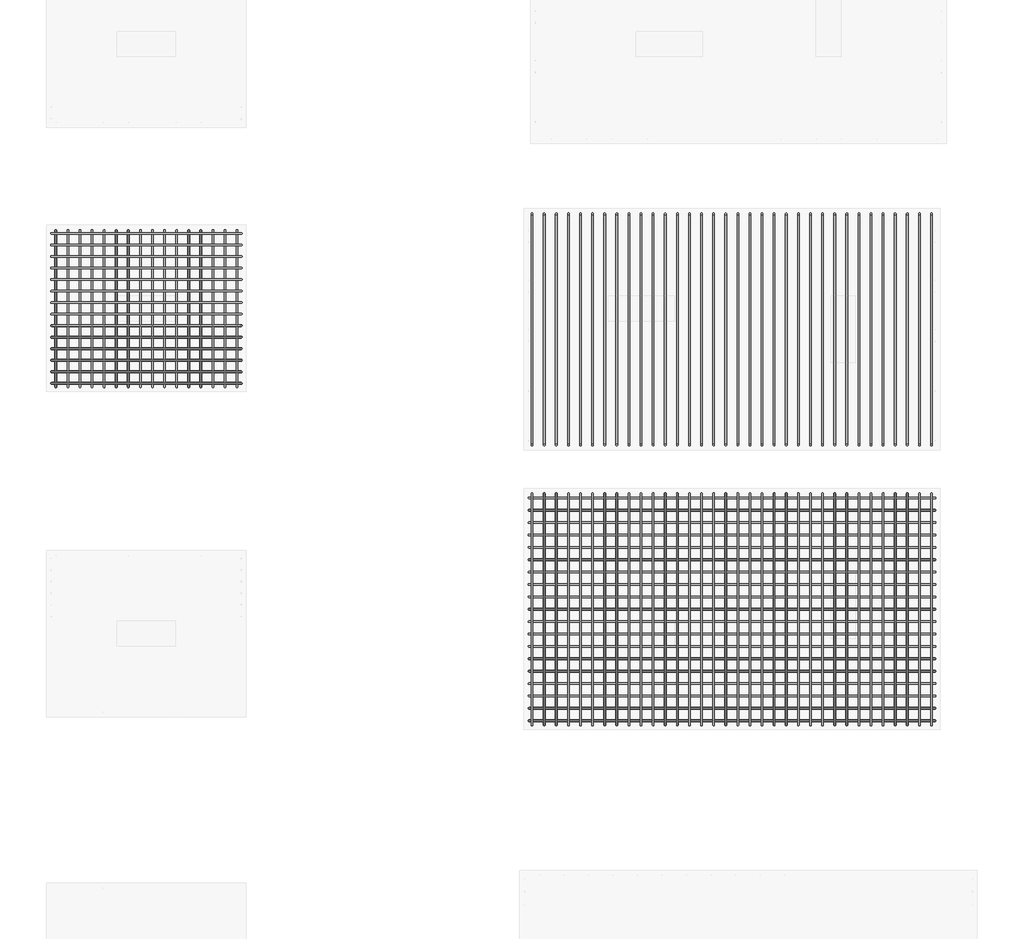
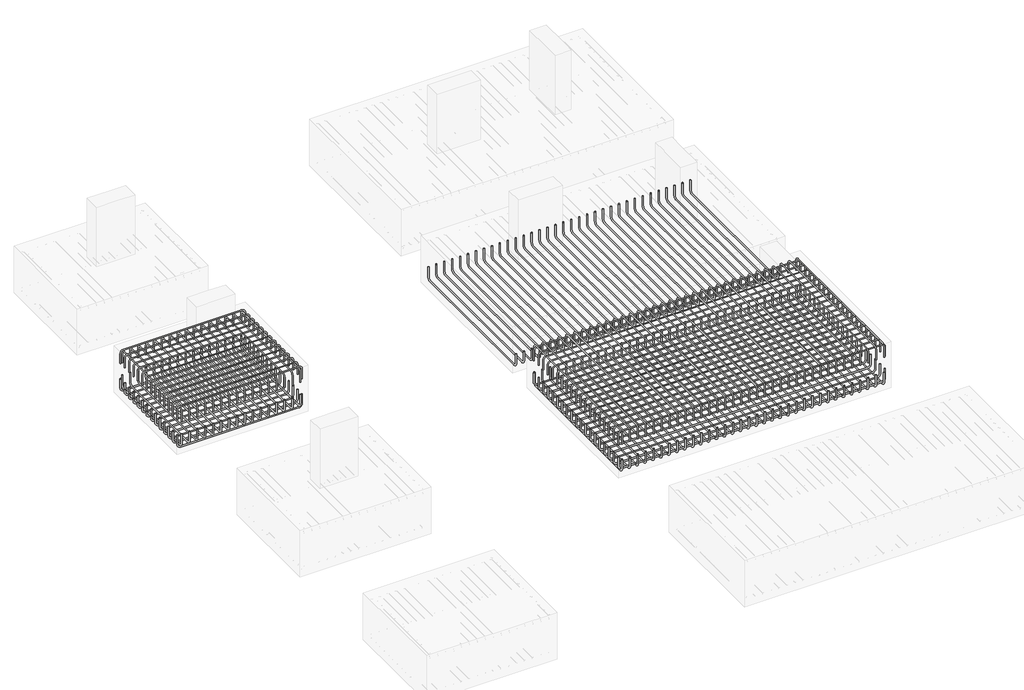
# One storey, part 10 of 21: 9 reinforcing bars.
"""IFC4 building model written with IfcOpenShell, lengths in millimetres."""

from ifc_helpers import new_model, si_unit, point, frame, origin, place, context, project, spatial, polyline, circle_curve, trimmed, segment, composite_curve, source, transform, mapped, element, save
from ifc_brep_helpers import swept_disk

model = new_model("IFC4")

# Units and contexts
model_context = context("Model", 3, world=origin())
ifc_project = project(units=[si_unit("LENGTHUNIT", "METRE", prefix="MILLI")], contexts=[model_context])

# Site, building, storey
site = spatial("IfcSite", under=ifc_project)
building = spatial("IfcBuilding", under=site)
storey = spatial("IfcBuildingStorey", under=building, Elevation=-1100.0)

# Reinforcing bars
placement = place(None, origin())
reinforcing_bar_shape = source(origin(), model_context, "Body", "SolidModel", [
    swept_disk(composite_curve([segment(polyline([(-23061.1351198, 8357.9216575, -1700.0), (-23061.1351198, 8357.9216575, -1882.5)]), True, "CONTINUOUS"), segment(trimmed(circle_curve(frame((-23118.6351198, 8357.9216575, -1882.5), z_axis=(0.0, 1.0, 0.0), x_axis=(57.5, 0.0, 0.0)), 57.5), [point((-23061.1351198, 8357.9216575, -1882.5))], [point((-23118.6351198, 8357.9216575, -1940.0))], True, "CARTESIAN"), True, "CONTINUOUS"), segment(polyline([(-23118.6351198, 8357.9216575, -1940.0), (-25283.6351198, 8357.9216575, -1940.0)]), True, "CONTINUOUS"), segment(trimmed(circle_curve(frame((-25283.6351198, 8357.9216575, -1882.5), z_axis=(0.0, 1.0, 0.0), x_axis=(0.0, 0.0, -57.5)), 57.5), [point((-25283.6351198, 8357.9216575, -1940.0))], [point((-25341.1351198, 8357.9216575, -1882.5))], True, "CARTESIAN"), True, "CONTINUOUS"), segment(polyline([(-25341.1351198, 8357.9216575, -1882.5), (-25341.1351198, 8357.9216575, -1700.0)]), True, "CONTINUOUS")], self_intersect=False), 10.0),
])
element("IfcReinforcingBar", 1, at=placement, inside=storey, context=model_context, shape_type="MappedRepresentation", body=[
    mapped(reinforcing_bar_shape, transform((0.0, 0.0, 0.0), x_axis=(1.0, 0.0, 0.0), y_axis=(0.0, 1.0, 0.0), z_axis=(0.0, 0.0, 1.0))),
    mapped(reinforcing_bar_shape, transform((0.0, -138.5928916, 0.0), x_axis=(1.0, 0.0, 0.0), y_axis=(0.0, 1.0, 0.0), z_axis=(0.0, 0.0, 1.0))),
    mapped(reinforcing_bar_shape, transform((0.0, -277.1857833, 0.0), x_axis=(1.0, 0.0, 0.0), y_axis=(0.0, 1.0, 0.0), z_axis=(0.0, 0.0, 1.0))),
    mapped(reinforcing_bar_shape, transform((0.0, -415.7786749, 0.0), x_axis=(1.0, 0.0, 0.0), y_axis=(0.0, 1.0, 0.0), z_axis=(0.0, 0.0, 1.0))),
    mapped(reinforcing_bar_shape, transform((0.0, -554.3715666, 0.0), x_axis=(1.0, 0.0, 0.0), y_axis=(0.0, 1.0, 0.0), z_axis=(0.0, 0.0, 1.0))),
    mapped(reinforcing_bar_shape, transform((0.0, -692.9644582, 0.0), x_axis=(1.0, 0.0, 0.0), y_axis=(0.0, 1.0, 0.0), z_axis=(0.0, 0.0, 1.0))),
    mapped(reinforcing_bar_shape, transform((0.0, -831.5573499, 0.0), x_axis=(1.0, 0.0, 0.0), y_axis=(0.0, 1.0, 0.0), z_axis=(0.0, 0.0, 1.0))),
    mapped(reinforcing_bar_shape, transform((0.0, -970.1502415, 0.0), x_axis=(1.0, 0.0, 0.0), y_axis=(0.0, 1.0, 0.0), z_axis=(0.0, 0.0, 1.0))),
    mapped(reinforcing_bar_shape, transform((0.0, -1108.7431331, 0.0), x_axis=(1.0, 0.0, 0.0), y_axis=(0.0, 1.0, 0.0), z_axis=(0.0, 0.0, 1.0))),
    mapped(reinforcing_bar_shape, transform((0.0, -1247.3360248, 0.0), x_axis=(1.0, 0.0, 0.0), y_axis=(0.0, 1.0, 0.0), z_axis=(0.0, 0.0, 1.0))),
    mapped(reinforcing_bar_shape, transform((0.0, -1385.9289164, 0.0), x_axis=(1.0, 0.0, 0.0), y_axis=(0.0, 1.0, 0.0), z_axis=(0.0, 0.0, 1.0))),
    mapped(reinforcing_bar_shape, transform((0.0, -1524.5218081, 0.0), x_axis=(1.0, 0.0, 0.0), y_axis=(0.0, 1.0, 0.0), z_axis=(0.0, 0.0, 1.0))),
    mapped(reinforcing_bar_shape, transform((0.0, -1663.1146997, 0.0), x_axis=(1.0, 0.0, 0.0), y_axis=(0.0, 1.0, 0.0), z_axis=(0.0, 0.0, 1.0))),
    mapped(reinforcing_bar_shape, transform((0.0, -1801.7075913, 0.0), x_axis=(1.0, 0.0, 0.0), y_axis=(0.0, 1.0, 0.0), z_axis=(0.0, 0.0, 1.0))),
])
reinforcing_bar_2_shape = source(origin(), model_context, "Body", "SolidModel", [
    swept_disk(composite_curve([segment(polyline([(-25343.1851198, 8357.9216575, -1400.0), (-25343.1851198, 8357.9216575, -1213.4)]), True, "CONTINUOUS"), segment(trimmed(circle_curve(frame((-25287.7351198, 8357.9216575, -1213.4), z_axis=(0.0, 1.0, 0.0), x_axis=(-55.45000000000073, 0.0, 0.0)), 55.45), [point((-25343.1851198, 8357.9216575, -1213.4))], [point((-25287.7351198, 8357.9216575, -1157.95))], True, "CARTESIAN"), True, "CONTINUOUS"), segment(polyline([(-25287.7351198, 8357.9216575, -1157.95), (-23114.5351198, 8357.9216575, -1157.95)]), True, "CONTINUOUS"), segment(trimmed(circle_curve(frame((-23114.5351198, 8357.9216575, -1213.4), z_axis=(0.0, 1.0, 0.0), x_axis=(0.0, 0.0, 55.450000000000045)), 55.45), [point((-23114.5351198, 8357.9216575, -1157.95))], [point((-23059.0851198, 8357.9216575, -1213.4))], True, "CARTESIAN"), True, "CONTINUOUS"), segment(polyline([(-23059.0851198, 8357.9216575, -1213.4), (-23059.0851198, 8357.9216575, -1400.0)]), True, "CONTINUOUS")], self_intersect=False), 7.95),
])
element("IfcReinforcingBar", 2, at=placement, inside=storey, context=model_context, shape_type="MappedRepresentation", body=[
    mapped(reinforcing_bar_2_shape, transform((0.0, 0.0, 0.0), x_axis=(1.0, 0.0, 0.0), y_axis=(0.0, 1.0, 0.0), z_axis=(0.0, 0.0, 1.0))),
    mapped(reinforcing_bar_2_shape, transform((0.0, -138.5928916, 0.0), x_axis=(1.0, 0.0, 0.0), y_axis=(0.0, 1.0, 0.0), z_axis=(0.0, 0.0, 1.0))),
    mapped(reinforcing_bar_2_shape, transform((0.0, -277.1857833, 0.0), x_axis=(1.0, 0.0, 0.0), y_axis=(0.0, 1.0, 0.0), z_axis=(0.0, 0.0, 1.0))),
    mapped(reinforcing_bar_2_shape, transform((0.0, -415.7786749, 0.0), x_axis=(1.0, 0.0, 0.0), y_axis=(0.0, 1.0, 0.0), z_axis=(0.0, 0.0, 1.0))),
    mapped(reinforcing_bar_2_shape, transform((0.0, -554.3715666, 0.0), x_axis=(1.0, 0.0, 0.0), y_axis=(0.0, 1.0, 0.0), z_axis=(0.0, 0.0, 1.0))),
    mapped(reinforcing_bar_2_shape, transform((0.0, -692.9644582, 0.0), x_axis=(1.0, 0.0, 0.0), y_axis=(0.0, 1.0, 0.0), z_axis=(0.0, 0.0, 1.0))),
    mapped(reinforcing_bar_2_shape, transform((0.0, -831.5573499, 0.0), x_axis=(1.0, 0.0, 0.0), y_axis=(0.0, 1.0, 0.0), z_axis=(0.0, 0.0, 1.0))),
    mapped(reinforcing_bar_2_shape, transform((0.0, -970.1502415, 0.0), x_axis=(1.0, 0.0, 0.0), y_axis=(0.0, 1.0, 0.0), z_axis=(0.0, 0.0, 1.0))),
    mapped(reinforcing_bar_2_shape, transform((0.0, -1108.7431331, 0.0), x_axis=(1.0, 0.0, 0.0), y_axis=(0.0, 1.0, 0.0), z_axis=(0.0, 0.0, 1.0))),
    mapped(reinforcing_bar_2_shape, transform((0.0, -1247.3360248, 0.0), x_axis=(1.0, 0.0, 0.0), y_axis=(0.0, 1.0, 0.0), z_axis=(0.0, 0.0, 1.0))),
    mapped(reinforcing_bar_2_shape, transform((0.0, -1385.9289164, 0.0), x_axis=(1.0, 0.0, 0.0), y_axis=(0.0, 1.0, 0.0), z_axis=(0.0, 0.0, 1.0))),
    mapped(reinforcing_bar_2_shape, transform((0.0, -1524.5218081, 0.0), x_axis=(1.0, 0.0, 0.0), y_axis=(0.0, 1.0, 0.0), z_axis=(0.0, 0.0, 1.0))),
    mapped(reinforcing_bar_2_shape, transform((0.0, -1663.1146997, 0.0), x_axis=(1.0, 0.0, 0.0), y_axis=(0.0, 1.0, 0.0), z_axis=(0.0, 0.0, 1.0))),
    mapped(reinforcing_bar_2_shape, transform((0.0, -1801.7075913, 0.0), x_axis=(1.0, 0.0, 0.0), y_axis=(0.0, 1.0, 0.0), z_axis=(0.0, 0.0, 1.0))),
])
reinforcing_bar_3_shape = source(origin(), model_context, "Body", "SolidModel", [
    swept_disk(composite_curve([segment(polyline([(-23110.9192838, 8396.2204288, -1428.1111113), (-23110.9192838, 8396.2204288, -1241.5111113)]), True, "CONTINUOUS"), segment(trimmed(circle_curve(frame((-23110.9192838, 8340.7704288, -1241.5111113), z_axis=(1.0, 0.0, 0.0), x_axis=(0.0, 55.44999999999891, 0.0)), 55.45), [point((-23110.9192838, 8396.2204288, -1241.5111113))], [point((-23110.9192838, 8340.7704288, -1186.0611113))], True, "CARTESIAN"), True, "CONTINUOUS"), segment(polyline([(-23110.9192838, 8340.7704288, -1186.0611113), (-23110.9192838, 6567.5704288, -1186.0611113)]), True, "CONTINUOUS"), segment(trimmed(circle_curve(frame((-23110.9192838, 6567.5704288, -1241.5111113), z_axis=(1.0, 0.0, 0.0), x_axis=(0.0, 0.0, 55.450000000000045)), 55.45), [point((-23110.9192838, 6567.5704288, -1186.0611113))], [point((-23110.9192838, 6512.1204288, -1241.5111113))], True, "CARTESIAN"), True, "CONTINUOUS"), segment(polyline([(-23110.9192838, 6512.1204288, -1241.5111113), (-23110.9192838, 6512.1204288, -1428.1111113)]), True, "CONTINUOUS")], self_intersect=False), 7.95),
])
element("IfcReinforcingBar", 3, at=placement, inside=storey, context=model_context, shape_type="MappedRepresentation", body=[
    mapped(reinforcing_bar_3_shape, transform((0.0, 0.0, 0.0), x_axis=(1.0, 0.0, 0.0), y_axis=(0.0, 1.0, 0.0), z_axis=(0.0, 0.0, 1.0))),
    mapped(reinforcing_bar_3_shape, transform((-145.2528929, 0.0, 0.0), x_axis=(1.0, 0.0, 0.0), y_axis=(0.0, 1.0, 0.0), z_axis=(0.0, 0.0, 1.0))),
    mapped(reinforcing_bar_3_shape, transform((-290.5057858, 0.0, 0.0), x_axis=(1.0, 0.0, 0.0), y_axis=(0.0, 1.0, 0.0), z_axis=(0.0, 0.0, 1.0))),
    mapped(reinforcing_bar_3_shape, transform((-435.7586787, 0.0, 0.0), x_axis=(1.0, 0.0, 0.0), y_axis=(0.0, 1.0, 0.0), z_axis=(0.0, 0.0, 1.0))),
    mapped(reinforcing_bar_3_shape, transform((-581.0115716, 0.0, 0.0), x_axis=(1.0, 0.0, 0.0), y_axis=(0.0, 1.0, 0.0), z_axis=(0.0, 0.0, 1.0))),
    mapped(reinforcing_bar_3_shape, transform((-726.2644645, 0.0, 0.0), x_axis=(1.0, 0.0, 0.0), y_axis=(0.0, 1.0, 0.0), z_axis=(0.0, 0.0, 1.0))),
    mapped(reinforcing_bar_3_shape, transform((-871.5173574, 0.0, 0.0), x_axis=(1.0, 0.0, 0.0), y_axis=(0.0, 1.0, 0.0), z_axis=(0.0, 0.0, 1.0))),
    mapped(reinforcing_bar_3_shape, transform((-1016.7702503, 0.0, 0.0), x_axis=(1.0, 0.0, 0.0), y_axis=(0.0, 1.0, 0.0), z_axis=(0.0, 0.0, 1.0))),
    mapped(reinforcing_bar_3_shape, transform((-1162.0231432, 0.0, 0.0), x_axis=(1.0, 0.0, 0.0), y_axis=(0.0, 1.0, 0.0), z_axis=(0.0, 0.0, 1.0))),
    mapped(reinforcing_bar_3_shape, transform((-1307.276036, 0.0, 0.0), x_axis=(1.0, 0.0, 0.0), y_axis=(0.0, 1.0, 0.0), z_axis=(0.0, 0.0, 1.0))),
    mapped(reinforcing_bar_3_shape, transform((-1452.5289289, 0.0, 0.0), x_axis=(1.0, 0.0, 0.0), y_axis=(0.0, 1.0, 0.0), z_axis=(0.0, 0.0, 1.0))),
    mapped(reinforcing_bar_3_shape, transform((-1597.7818218, 0.0, 0.0), x_axis=(1.0, 0.0, 0.0), y_axis=(0.0, 1.0, 0.0), z_axis=(0.0, 0.0, 1.0))),
    mapped(reinforcing_bar_3_shape, transform((-1743.0347147, 0.0, 0.0), x_axis=(1.0, 0.0, 0.0), y_axis=(0.0, 1.0, 0.0), z_axis=(0.0, 0.0, 1.0))),
    mapped(reinforcing_bar_3_shape, transform((-1888.2876076, 0.0, 0.0), x_axis=(1.0, 0.0, 0.0), y_axis=(0.0, 1.0, 0.0), z_axis=(0.0, 0.0, 1.0))),
    mapped(reinforcing_bar_3_shape, transform((-2033.5405005, 0.0, 0.0), x_axis=(1.0, 0.0, 0.0), y_axis=(0.0, 1.0, 0.0), z_axis=(0.0, 0.0, 1.0))),
    mapped(reinforcing_bar_3_shape, transform((-2178.7933934, 0.0, 0.0), x_axis=(1.0, 0.0, 0.0), y_axis=(0.0, 1.0, 0.0), z_axis=(0.0, 0.0, 1.0))),
])
reinforcing_bar_4_shape = source(origin(), model_context, "Body", "SolidModel", [
    swept_disk(composite_curve([segment(polyline([(-25289.7126773, 8394.1704288, -1669.8442859), (-25289.7126773, 8394.1704288, -1852.3442859)]), True, "CONTINUOUS"), segment(trimmed(circle_curve(frame((-25289.7126773, 8336.6704288, -1852.3442859), z_axis=(-1.0, 0.0, 0.0), x_axis=(0.0, 57.5, 0.0)), 57.5), [point((-25289.7126773, 8394.1704288, -1852.3442859))], [point((-25289.7126773, 8336.6704288, -1909.8442859))], True, "CARTESIAN"), True, "CONTINUOUS"), segment(polyline([(-25289.7126773, 8336.6704288, -1909.8442859), (-25289.7126773, 6571.6704288, -1909.8442859)]), True, "CONTINUOUS"), segment(trimmed(circle_curve(frame((-25289.7126773, 6571.6704288, -1852.3442859), z_axis=(-1.0, 0.0, 0.0), x_axis=(0.0, 0.0, -57.5)), 57.5), [point((-25289.7126773, 6571.6704288, -1909.8442859))], [point((-25289.7126773, 6514.1704288, -1852.3442859))], True, "CARTESIAN"), True, "CONTINUOUS"), segment(polyline([(-25289.7126773, 6514.1704288, -1852.3442859), (-25289.7126773, 6514.1704288, -1669.8442859)]), True, "CONTINUOUS")], self_intersect=False), 10.0),
])
element("IfcReinforcingBar", 4, at=placement, inside=storey, context=model_context, shape_type="MappedRepresentation", body=[
    mapped(reinforcing_bar_4_shape, transform((0.0, 0.0, 0.0), x_axis=(1.0, 0.0, 0.0), y_axis=(0.0, 1.0, 0.0), z_axis=(0.0, 0.0, 1.0))),
    mapped(reinforcing_bar_4_shape, transform((145.2528929, 0.0, 0.0), x_axis=(1.0, 0.0, 0.0), y_axis=(0.0, 1.0, 0.0), z_axis=(0.0, 0.0, 1.0))),
    mapped(reinforcing_bar_4_shape, transform((290.5057858, 0.0, 0.0), x_axis=(1.0, 0.0, 0.0), y_axis=(0.0, 1.0, 0.0), z_axis=(0.0, 0.0, 1.0))),
    mapped(reinforcing_bar_4_shape, transform((435.7586787, 0.0, 0.0), x_axis=(1.0, 0.0, 0.0), y_axis=(0.0, 1.0, 0.0), z_axis=(0.0, 0.0, 1.0))),
    mapped(reinforcing_bar_4_shape, transform((581.0115716, 0.0, 0.0), x_axis=(1.0, 0.0, 0.0), y_axis=(0.0, 1.0, 0.0), z_axis=(0.0, 0.0, 1.0))),
    mapped(reinforcing_bar_4_shape, transform((726.2644645, 0.0, 0.0), x_axis=(1.0, 0.0, 0.0), y_axis=(0.0, 1.0, 0.0), z_axis=(0.0, 0.0, 1.0))),
    mapped(reinforcing_bar_4_shape, transform((871.5173574, 0.0, 0.0), x_axis=(1.0, 0.0, 0.0), y_axis=(0.0, 1.0, 0.0), z_axis=(0.0, 0.0, 1.0))),
    mapped(reinforcing_bar_4_shape, transform((1016.7702503, 0.0, 0.0), x_axis=(1.0, 0.0, 0.0), y_axis=(0.0, 1.0, 0.0), z_axis=(0.0, 0.0, 1.0))),
    mapped(reinforcing_bar_4_shape, transform((1162.0231432, 0.0, 0.0), x_axis=(1.0, 0.0, 0.0), y_axis=(0.0, 1.0, 0.0), z_axis=(0.0, 0.0, 1.0))),
    mapped(reinforcing_bar_4_shape, transform((1307.276036, 0.0, 0.0), x_axis=(1.0, 0.0, 0.0), y_axis=(0.0, 1.0, 0.0), z_axis=(0.0, 0.0, 1.0))),
    mapped(reinforcing_bar_4_shape, transform((1452.5289289, 0.0, 0.0), x_axis=(1.0, 0.0, 0.0), y_axis=(0.0, 1.0, 0.0), z_axis=(0.0, 0.0, 1.0))),
    mapped(reinforcing_bar_4_shape, transform((1597.7818218, 0.0, 0.0), x_axis=(1.0, 0.0, 0.0), y_axis=(0.0, 1.0, 0.0), z_axis=(0.0, 0.0, 1.0))),
    mapped(reinforcing_bar_4_shape, transform((1743.0347147, 0.0, 0.0), x_axis=(1.0, 0.0, 0.0), y_axis=(0.0, 1.0, 0.0), z_axis=(0.0, 0.0, 1.0))),
    mapped(reinforcing_bar_4_shape, transform((1888.2876076, 0.0, 0.0), x_axis=(1.0, 0.0, 0.0), y_axis=(0.0, 1.0, 0.0), z_axis=(0.0, 0.0, 1.0))),
    mapped(reinforcing_bar_4_shape, transform((2033.5405005, 0.0, 0.0), x_axis=(1.0, 0.0, 0.0), y_axis=(0.0, 1.0, 0.0), z_axis=(0.0, 0.0, 1.0))),
    mapped(reinforcing_bar_4_shape, transform((2178.7933934, 0.0, 0.0), x_axis=(1.0, 0.0, 0.0), y_axis=(0.0, 1.0, 0.0), z_axis=(0.0, 0.0, 1.0))),
])
reinforcing_bar_5_shape = source(origin(), model_context, "Body", "SolidModel", [
    swept_disk(composite_curve([segment(polyline([(-19564.5839151, 5229.1704288, -1700.0), (-19564.5839151, 5229.1704288, -1882.5)]), True, "CONTINUOUS"), segment(trimmed(circle_curve(frame((-19564.5839151, 5171.6704288, -1882.5), z_axis=(-1.0, 0.0, 0.0), x_axis=(0.0, 57.5, 0.0)), 57.5), [point((-19564.5839151, 5229.1704288, -1882.5))], [point((-19564.5839151, 5171.6704288, -1940.0))], True, "CARTESIAN"), True, "CONTINUOUS"), segment(polyline([(-19564.5839151, 5171.6704288, -1940.0), (-19564.5839151, 2506.6704288, -1940.0)]), True, "CONTINUOUS"), segment(trimmed(circle_curve(frame((-19564.5839151, 2506.6704288, -1882.5), z_axis=(-1.0, 0.0, 0.0), x_axis=(0.0, 0.0, -57.5)), 57.5), [point((-19564.5839151, 2506.6704288, -1940.0))], [point((-19564.5839151, 2449.1704288, -1882.5))], True, "CARTESIAN"), True, "CONTINUOUS"), segment(polyline([(-19564.5839151, 2449.1704288, -1882.5), (-19564.5839151, 2449.1704288, -1700.0)]), True, "CONTINUOUS")], self_intersect=False), 10.0),
])
element("IfcReinforcingBar", 5, at=placement, inside=storey, context=model_context, shape_type="MappedRepresentation", body=[
    mapped(reinforcing_bar_5_shape, transform((0.0, 0.0, 0.0), x_axis=(1.0, 0.0, 0.0), y_axis=(0.0, 1.0, 0.0), z_axis=(0.0, 0.0, 1.0))),
    mapped(reinforcing_bar_5_shape, transform((145.5062906, 0.0, 0.0), x_axis=(1.0, 0.0, 0.0), y_axis=(0.0, 1.0, 0.0), z_axis=(0.0, 0.0, 1.0))),
    mapped(reinforcing_bar_5_shape, transform((291.0125813, 0.0, 0.0), x_axis=(1.0, 0.0, 0.0), y_axis=(0.0, 1.0, 0.0), z_axis=(0.0, 0.0, 1.0))),
    mapped(reinforcing_bar_5_shape, transform((436.5188719, 0.0, 0.0), x_axis=(1.0, 0.0, 0.0), y_axis=(0.0, 1.0, 0.0), z_axis=(0.0, 0.0, 1.0))),
    mapped(reinforcing_bar_5_shape, transform((582.0251626, 0.0, 0.0), x_axis=(1.0, 0.0, 0.0), y_axis=(0.0, 1.0, 0.0), z_axis=(0.0, 0.0, 1.0))),
    mapped(reinforcing_bar_5_shape, transform((727.5314532, 0.0, 0.0), x_axis=(1.0, 0.0, 0.0), y_axis=(0.0, 1.0, 0.0), z_axis=(0.0, 0.0, 1.0))),
    mapped(reinforcing_bar_5_shape, transform((873.0377439, 0.0, 0.0), x_axis=(1.0, 0.0, 0.0), y_axis=(0.0, 1.0, 0.0), z_axis=(0.0, 0.0, 1.0))),
    mapped(reinforcing_bar_5_shape, transform((1018.5440345, 0.0, 0.0), x_axis=(1.0, 0.0, 0.0), y_axis=(0.0, 1.0, 0.0), z_axis=(0.0, 0.0, 1.0))),
    mapped(reinforcing_bar_5_shape, transform((1164.0503252, 0.0, 0.0), x_axis=(1.0, 0.0, 0.0), y_axis=(0.0, 1.0, 0.0), z_axis=(0.0, 0.0, 1.0))),
    mapped(reinforcing_bar_5_shape, transform((1309.5566158, 0.0, 0.0), x_axis=(1.0, 0.0, 0.0), y_axis=(0.0, 1.0, 0.0), z_axis=(0.0, 0.0, 1.0))),
    mapped(reinforcing_bar_5_shape, transform((1455.0629065, 0.0, 0.0), x_axis=(1.0, 0.0, 0.0), y_axis=(0.0, 1.0, 0.0), z_axis=(0.0, 0.0, 1.0))),
    mapped(reinforcing_bar_5_shape, transform((1600.5691971, 0.0, 0.0), x_axis=(1.0, 0.0, 0.0), y_axis=(0.0, 1.0, 0.0), z_axis=(0.0, 0.0, 1.0))),
    mapped(reinforcing_bar_5_shape, transform((1746.0754878, 0.0, 0.0), x_axis=(1.0, 0.0, 0.0), y_axis=(0.0, 1.0, 0.0), z_axis=(0.0, 0.0, 1.0))),
    mapped(reinforcing_bar_5_shape, transform((1891.5817784, 0.0, 0.0), x_axis=(1.0, 0.0, 0.0), y_axis=(0.0, 1.0, 0.0), z_axis=(0.0, 0.0, 1.0))),
    mapped(reinforcing_bar_5_shape, transform((2037.0880691, 0.0, 0.0), x_axis=(1.0, 0.0, 0.0), y_axis=(0.0, 1.0, 0.0), z_axis=(0.0, 0.0, 1.0))),
    mapped(reinforcing_bar_5_shape, transform((2182.5943597, 0.0, 0.0), x_axis=(1.0, 0.0, 0.0), y_axis=(0.0, 1.0, 0.0), z_axis=(0.0, 0.0, 1.0))),
    mapped(reinforcing_bar_5_shape, transform((2328.1006504, 0.0, 0.0), x_axis=(1.0, 0.0, 0.0), y_axis=(0.0, 1.0, 0.0), z_axis=(0.0, 0.0, 1.0))),
    mapped(reinforcing_bar_5_shape, transform((2473.606941, 0.0, 0.0), x_axis=(1.0, 0.0, 0.0), y_axis=(0.0, 1.0, 0.0), z_axis=(0.0, 0.0, 1.0))),
    mapped(reinforcing_bar_5_shape, transform((2619.1132316, 0.0, 0.0), x_axis=(1.0, 0.0, 0.0), y_axis=(0.0, 1.0, 0.0), z_axis=(0.0, 0.0, 1.0))),
    mapped(reinforcing_bar_5_shape, transform((2764.6195223, 0.0, 0.0), x_axis=(1.0, 0.0, 0.0), y_axis=(0.0, 1.0, 0.0), z_axis=(0.0, 0.0, 1.0))),
    mapped(reinforcing_bar_5_shape, transform((2910.1258129, 0.0, 0.0), x_axis=(1.0, 0.0, 0.0), y_axis=(0.0, 1.0, 0.0), z_axis=(0.0, 0.0, 1.0))),
    mapped(reinforcing_bar_5_shape, transform((3055.6321036, 0.0, 0.0), x_axis=(1.0, 0.0, 0.0), y_axis=(0.0, 1.0, 0.0), z_axis=(0.0, 0.0, 1.0))),
    mapped(reinforcing_bar_5_shape, transform((3201.1383942, 0.0, 0.0), x_axis=(1.0, 0.0, 0.0), y_axis=(0.0, 1.0, 0.0), z_axis=(0.0, 0.0, 1.0))),
    mapped(reinforcing_bar_5_shape, transform((3346.6446849, 0.0, 0.0), x_axis=(1.0, 0.0, 0.0), y_axis=(0.0, 1.0, 0.0), z_axis=(0.0, 0.0, 1.0))),
    mapped(reinforcing_bar_5_shape, transform((3492.1509755, 0.0, 0.0), x_axis=(1.0, 0.0, 0.0), y_axis=(0.0, 1.0, 0.0), z_axis=(0.0, 0.0, 1.0))),
    mapped(reinforcing_bar_5_shape, transform((3637.6572662, 0.0, 0.0), x_axis=(1.0, 0.0, 0.0), y_axis=(0.0, 1.0, 0.0), z_axis=(0.0, 0.0, 1.0))),
    mapped(reinforcing_bar_5_shape, transform((3783.1635568, 0.0, 0.0), x_axis=(1.0, 0.0, 0.0), y_axis=(0.0, 1.0, 0.0), z_axis=(0.0, 0.0, 1.0))),
    mapped(reinforcing_bar_5_shape, transform((3928.6698475, 0.0, 0.0), x_axis=(1.0, 0.0, 0.0), y_axis=(0.0, 1.0, 0.0), z_axis=(0.0, 0.0, 1.0))),
    mapped(reinforcing_bar_5_shape, transform((4074.1761381, 0.0, 0.0), x_axis=(1.0, 0.0, 0.0), y_axis=(0.0, 1.0, 0.0), z_axis=(0.0, 0.0, 1.0))),
    mapped(reinforcing_bar_5_shape, transform((4219.6824288, 0.0, 0.0), x_axis=(1.0, 0.0, 0.0), y_axis=(0.0, 1.0, 0.0), z_axis=(0.0, 0.0, 1.0))),
    mapped(reinforcing_bar_5_shape, transform((4365.1887194, 0.0, 0.0), x_axis=(1.0, 0.0, 0.0), y_axis=(0.0, 1.0, 0.0), z_axis=(0.0, 0.0, 1.0))),
    mapped(reinforcing_bar_5_shape, transform((4510.6950101, 0.0, 0.0), x_axis=(1.0, 0.0, 0.0), y_axis=(0.0, 1.0, 0.0), z_axis=(0.0, 0.0, 1.0))),
    mapped(reinforcing_bar_5_shape, transform((4656.2013007, 0.0, 0.0), x_axis=(1.0, 0.0, 0.0), y_axis=(0.0, 1.0, 0.0), z_axis=(0.0, 0.0, 1.0))),
    mapped(reinforcing_bar_5_shape, transform((4801.7075913, 0.0, 0.0), x_axis=(1.0, 0.0, 0.0), y_axis=(0.0, 1.0, 0.0), z_axis=(0.0, 0.0, 1.0))),
])
reinforcing_bar_6_shape = source(origin(), model_context, "Body", "SolidModel", [
    swept_disk(composite_curve([segment(polyline([(-19564.5839151, 2447.1204288, -1400.0), (-19564.5839151, 2447.1204288, -1213.4)]), True, "CONTINUOUS"), segment(trimmed(circle_curve(frame((-19564.5839151, 2502.5704288, -1213.4), z_axis=(-1.0, 0.0, 0.0), x_axis=(0.0, -55.45000000000027, 0.0)), 55.45), [point((-19564.5839151, 2447.1204288, -1213.4))], [point((-19564.5839151, 2502.5704288, -1157.95))], True, "CARTESIAN"), True, "CONTINUOUS"), segment(polyline([(-19564.5839151, 2502.5704288, -1157.95), (-19564.5839151, 5175.7704288, -1157.95)]), True, "CONTINUOUS"), segment(trimmed(circle_curve(frame((-19564.5839151, 5175.7704288, -1213.4), z_axis=(-1.0, 0.0, 0.0), x_axis=(0.0, 0.0, 55.450000000000045)), 55.45), [point((-19564.5839151, 5175.7704288, -1157.95))], [point((-19564.5839151, 5231.2204288, -1213.4))], True, "CARTESIAN"), True, "CONTINUOUS"), segment(polyline([(-19564.5839151, 5231.2204288, -1213.4), (-19564.5839151, 5231.2204288, -1400.0)]), True, "CONTINUOUS")], self_intersect=False), 7.95),
])
element("IfcReinforcingBar", 6, at=placement, inside=storey, context=model_context, shape_type="MappedRepresentation", body=[
    mapped(reinforcing_bar_6_shape, transform((0.0, 0.0, 0.0), x_axis=(1.0, 0.0, 0.0), y_axis=(0.0, 1.0, 0.0), z_axis=(0.0, 0.0, 1.0))),
    mapped(reinforcing_bar_6_shape, transform((145.5062906, 0.0, 0.0), x_axis=(1.0, 0.0, 0.0), y_axis=(0.0, 1.0, 0.0), z_axis=(0.0, 0.0, 1.0))),
    mapped(reinforcing_bar_6_shape, transform((291.0125813, 0.0, 0.0), x_axis=(1.0, 0.0, 0.0), y_axis=(0.0, 1.0, 0.0), z_axis=(0.0, 0.0, 1.0))),
    mapped(reinforcing_bar_6_shape, transform((436.5188719, 0.0, 0.0), x_axis=(1.0, 0.0, 0.0), y_axis=(0.0, 1.0, 0.0), z_axis=(0.0, 0.0, 1.0))),
    mapped(reinforcing_bar_6_shape, transform((582.0251626, 0.0, 0.0), x_axis=(1.0, 0.0, 0.0), y_axis=(0.0, 1.0, 0.0), z_axis=(0.0, 0.0, 1.0))),
    mapped(reinforcing_bar_6_shape, transform((727.5314532, 0.0, 0.0), x_axis=(1.0, 0.0, 0.0), y_axis=(0.0, 1.0, 0.0), z_axis=(0.0, 0.0, 1.0))),
    mapped(reinforcing_bar_6_shape, transform((873.0377439, 0.0, 0.0), x_axis=(1.0, 0.0, 0.0), y_axis=(0.0, 1.0, 0.0), z_axis=(0.0, 0.0, 1.0))),
    mapped(reinforcing_bar_6_shape, transform((1018.5440345, 0.0, 0.0), x_axis=(1.0, 0.0, 0.0), y_axis=(0.0, 1.0, 0.0), z_axis=(0.0, 0.0, 1.0))),
    mapped(reinforcing_bar_6_shape, transform((1164.0503252, 0.0, 0.0), x_axis=(1.0, 0.0, 0.0), y_axis=(0.0, 1.0, 0.0), z_axis=(0.0, 0.0, 1.0))),
    mapped(reinforcing_bar_6_shape, transform((1309.5566158, 0.0, 0.0), x_axis=(1.0, 0.0, 0.0), y_axis=(0.0, 1.0, 0.0), z_axis=(0.0, 0.0, 1.0))),
    mapped(reinforcing_bar_6_shape, transform((1455.0629065, 0.0, 0.0), x_axis=(1.0, 0.0, 0.0), y_axis=(0.0, 1.0, 0.0), z_axis=(0.0, 0.0, 1.0))),
    mapped(reinforcing_bar_6_shape, transform((1600.5691971, 0.0, 0.0), x_axis=(1.0, 0.0, 0.0), y_axis=(0.0, 1.0, 0.0), z_axis=(0.0, 0.0, 1.0))),
    mapped(reinforcing_bar_6_shape, transform((1746.0754878, 0.0, 0.0), x_axis=(1.0, 0.0, 0.0), y_axis=(0.0, 1.0, 0.0), z_axis=(0.0, 0.0, 1.0))),
    mapped(reinforcing_bar_6_shape, transform((1891.5817784, 0.0, 0.0), x_axis=(1.0, 0.0, 0.0), y_axis=(0.0, 1.0, 0.0), z_axis=(0.0, 0.0, 1.0))),
    mapped(reinforcing_bar_6_shape, transform((2037.0880691, 0.0, 0.0), x_axis=(1.0, 0.0, 0.0), y_axis=(0.0, 1.0, 0.0), z_axis=(0.0, 0.0, 1.0))),
    mapped(reinforcing_bar_6_shape, transform((2182.5943597, 0.0, 0.0), x_axis=(1.0, 0.0, 0.0), y_axis=(0.0, 1.0, 0.0), z_axis=(0.0, 0.0, 1.0))),
    mapped(reinforcing_bar_6_shape, transform((2328.1006504, 0.0, 0.0), x_axis=(1.0, 0.0, 0.0), y_axis=(0.0, 1.0, 0.0), z_axis=(0.0, 0.0, 1.0))),
    mapped(reinforcing_bar_6_shape, transform((2473.606941, 0.0, 0.0), x_axis=(1.0, 0.0, 0.0), y_axis=(0.0, 1.0, 0.0), z_axis=(0.0, 0.0, 1.0))),
    mapped(reinforcing_bar_6_shape, transform((2619.1132316, 0.0, 0.0), x_axis=(1.0, 0.0, 0.0), y_axis=(0.0, 1.0, 0.0), z_axis=(0.0, 0.0, 1.0))),
    mapped(reinforcing_bar_6_shape, transform((2764.6195223, 0.0, 0.0), x_axis=(1.0, 0.0, 0.0), y_axis=(0.0, 1.0, 0.0), z_axis=(0.0, 0.0, 1.0))),
    mapped(reinforcing_bar_6_shape, transform((2910.1258129, 0.0, 0.0), x_axis=(1.0, 0.0, 0.0), y_axis=(0.0, 1.0, 0.0), z_axis=(0.0, 0.0, 1.0))),
    mapped(reinforcing_bar_6_shape, transform((3055.6321036, 0.0, 0.0), x_axis=(1.0, 0.0, 0.0), y_axis=(0.0, 1.0, 0.0), z_axis=(0.0, 0.0, 1.0))),
    mapped(reinforcing_bar_6_shape, transform((3201.1383942, 0.0, 0.0), x_axis=(1.0, 0.0, 0.0), y_axis=(0.0, 1.0, 0.0), z_axis=(0.0, 0.0, 1.0))),
    mapped(reinforcing_bar_6_shape, transform((3346.6446849, 0.0, 0.0), x_axis=(1.0, 0.0, 0.0), y_axis=(0.0, 1.0, 0.0), z_axis=(0.0, 0.0, 1.0))),
    mapped(reinforcing_bar_6_shape, transform((3492.1509755, 0.0, 0.0), x_axis=(1.0, 0.0, 0.0), y_axis=(0.0, 1.0, 0.0), z_axis=(0.0, 0.0, 1.0))),
    mapped(reinforcing_bar_6_shape, transform((3637.6572662, 0.0, 0.0), x_axis=(1.0, 0.0, 0.0), y_axis=(0.0, 1.0, 0.0), z_axis=(0.0, 0.0, 1.0))),
    mapped(reinforcing_bar_6_shape, transform((3783.1635568, 0.0, 0.0), x_axis=(1.0, 0.0, 0.0), y_axis=(0.0, 1.0, 0.0), z_axis=(0.0, 0.0, 1.0))),
    mapped(reinforcing_bar_6_shape, transform((3928.6698475, 0.0, 0.0), x_axis=(1.0, 0.0, 0.0), y_axis=(0.0, 1.0, 0.0), z_axis=(0.0, 0.0, 1.0))),
    mapped(reinforcing_bar_6_shape, transform((4074.1761381, 0.0, 0.0), x_axis=(1.0, 0.0, 0.0), y_axis=(0.0, 1.0, 0.0), z_axis=(0.0, 0.0, 1.0))),
    mapped(reinforcing_bar_6_shape, transform((4219.6824288, 0.0, 0.0), x_axis=(1.0, 0.0, 0.0), y_axis=(0.0, 1.0, 0.0), z_axis=(0.0, 0.0, 1.0))),
    mapped(reinforcing_bar_6_shape, transform((4365.1887194, 0.0, 0.0), x_axis=(1.0, 0.0, 0.0), y_axis=(0.0, 1.0, 0.0), z_axis=(0.0, 0.0, 1.0))),
    mapped(reinforcing_bar_6_shape, transform((4510.6950101, 0.0, 0.0), x_axis=(1.0, 0.0, 0.0), y_axis=(0.0, 1.0, 0.0), z_axis=(0.0, 0.0, 1.0))),
    mapped(reinforcing_bar_6_shape, transform((4656.2013007, 0.0, 0.0), x_axis=(1.0, 0.0, 0.0), y_axis=(0.0, 1.0, 0.0), z_axis=(0.0, 0.0, 1.0))),
    mapped(reinforcing_bar_6_shape, transform((4801.7075913, 0.0, 0.0), x_axis=(1.0, 0.0, 0.0), y_axis=(0.0, 1.0, 0.0), z_axis=(0.0, 0.0, 1.0))),
])
reinforcing_bar_7_shape = source(origin(), model_context, "Body", "SolidModel", [
    swept_disk(composite_curve([segment(polyline([(-19602.8826863, 5179.3862648, -1428.1111113), (-19602.8826863, 5179.3862648, -1241.5111113)]), True, "CONTINUOUS"), segment(trimmed(circle_curve(frame((-19547.4326863, 5179.3862648, -1241.5111113), z_axis=(0.0, 1.0, 0.0), x_axis=(-55.45000000000073, 0.0, 0.0)), 55.45), [point((-19602.8826863, 5179.3862648, -1241.5111113))], [point((-19547.4326863, 5179.3862648, -1186.0611113))], True, "CARTESIAN"), True, "CONTINUOUS"), segment(polyline([(-19547.4326863, 5179.3862648, -1186.0611113), (-14774.2326863, 5179.3862648, -1186.0611113)]), True, "CONTINUOUS"), segment(trimmed(circle_curve(frame((-14774.2326863, 5179.3862648, -1241.5111113), z_axis=(0.0, 1.0, 0.0), x_axis=(0.0, 0.0, 55.450000000000045)), 55.45), [point((-14774.2326863, 5179.3862648, -1186.0611113))], [point((-14718.7826863, 5179.3862648, -1241.5111113))], True, "CARTESIAN"), True, "CONTINUOUS"), segment(polyline([(-14718.7826863, 5179.3862648, -1241.5111113), (-14718.7826863, 5179.3862648, -1428.1111113)]), True, "CONTINUOUS")], self_intersect=False), 7.95),
])
element("IfcReinforcingBar", 7, at=placement, inside=storey, context=model_context, shape_type="MappedRepresentation", body=[
    mapped(reinforcing_bar_7_shape, transform((0.0, 0.0, 0.0), x_axis=(1.0, 0.0, 0.0), y_axis=(0.0, 1.0, 0.0), z_axis=(0.0, 0.0, 1.0))),
    mapped(reinforcing_bar_7_shape, transform((0.0, -148.8218552, 0.0), x_axis=(1.0, 0.0, 0.0), y_axis=(0.0, 1.0, 0.0), z_axis=(0.0, 0.0, 1.0))),
    mapped(reinforcing_bar_7_shape, transform((0.0, -297.6437104, 0.0), x_axis=(1.0, 0.0, 0.0), y_axis=(0.0, 1.0, 0.0), z_axis=(0.0, 0.0, 1.0))),
    mapped(reinforcing_bar_7_shape, transform((0.0, -446.4655656, 0.0), x_axis=(1.0, 0.0, 0.0), y_axis=(0.0, 1.0, 0.0), z_axis=(0.0, 0.0, 1.0))),
    mapped(reinforcing_bar_7_shape, transform((0.0, -595.2874208, 0.0), x_axis=(1.0, 0.0, 0.0), y_axis=(0.0, 1.0, 0.0), z_axis=(0.0, 0.0, 1.0))),
    mapped(reinforcing_bar_7_shape, transform((0.0, -744.1092759, 0.0), x_axis=(1.0, 0.0, 0.0), y_axis=(0.0, 1.0, 0.0), z_axis=(0.0, 0.0, 1.0))),
    mapped(reinforcing_bar_7_shape, transform((0.0, -892.9311311, 0.0), x_axis=(1.0, 0.0, 0.0), y_axis=(0.0, 1.0, 0.0), z_axis=(0.0, 0.0, 1.0))),
    mapped(reinforcing_bar_7_shape, transform((0.0, -1041.7529863, 0.0), x_axis=(1.0, 0.0, 0.0), y_axis=(0.0, 1.0, 0.0), z_axis=(0.0, 0.0, 1.0))),
    mapped(reinforcing_bar_7_shape, transform((0.0, -1190.5748415, 0.0), x_axis=(1.0, 0.0, 0.0), y_axis=(0.0, 1.0, 0.0), z_axis=(0.0, 0.0, 1.0))),
    mapped(reinforcing_bar_7_shape, transform((0.0, -1339.3966967, 0.0), x_axis=(1.0, 0.0, 0.0), y_axis=(0.0, 1.0, 0.0), z_axis=(0.0, 0.0, 1.0))),
    mapped(reinforcing_bar_7_shape, transform((0.0, -1488.2185519, 0.0), x_axis=(1.0, 0.0, 0.0), y_axis=(0.0, 1.0, 0.0), z_axis=(0.0, 0.0, 1.0))),
    mapped(reinforcing_bar_7_shape, transform((0.0, -1637.0404071, 0.0), x_axis=(1.0, 0.0, 0.0), y_axis=(0.0, 1.0, 0.0), z_axis=(0.0, 0.0, 1.0))),
    mapped(reinforcing_bar_7_shape, transform((0.0, -1785.8622623, 0.0), x_axis=(1.0, 0.0, 0.0), y_axis=(0.0, 1.0, 0.0), z_axis=(0.0, 0.0, 1.0))),
    mapped(reinforcing_bar_7_shape, transform((0.0, -1934.6841175, 0.0), x_axis=(1.0, 0.0, 0.0), y_axis=(0.0, 1.0, 0.0), z_axis=(0.0, 0.0, 1.0))),
    mapped(reinforcing_bar_7_shape, transform((0.0, -2083.5059727, 0.0), x_axis=(1.0, 0.0, 0.0), y_axis=(0.0, 1.0, 0.0), z_axis=(0.0, 0.0, 1.0))),
    mapped(reinforcing_bar_7_shape, transform((0.0, -2232.3278278, 0.0), x_axis=(1.0, 0.0, 0.0), y_axis=(0.0, 1.0, 0.0), z_axis=(0.0, 0.0, 1.0))),
    mapped(reinforcing_bar_7_shape, transform((0.0, -2381.149683, 0.0), x_axis=(1.0, 0.0, 0.0), y_axis=(0.0, 1.0, 0.0), z_axis=(0.0, 0.0, 1.0))),
    mapped(reinforcing_bar_7_shape, transform((0.0, -2529.9715382, 0.0), x_axis=(1.0, 0.0, 0.0), y_axis=(0.0, 1.0, 0.0), z_axis=(0.0, 0.0, 1.0))),
    mapped(reinforcing_bar_7_shape, transform((0.0, -2678.7933934, 0.0), x_axis=(1.0, 0.0, 0.0), y_axis=(0.0, 1.0, 0.0), z_axis=(0.0, 0.0, 1.0))),
])
reinforcing_bar_8_shape = source(origin(), model_context, "Body", "SolidModel", [
    swept_disk(composite_curve([segment(polyline([(-19600.8326863, 2500.5928714, -1669.8442859), (-19600.8326863, 2500.5928714, -1852.3442859)]), True, "CONTINUOUS"), segment(trimmed(circle_curve(frame((-19543.3326863, 2500.5928714, -1852.3442859), z_axis=(0.0, -1.0, 0.0), x_axis=(-57.5, 0.0, 0.0)), 57.5), [point((-19600.8326863, 2500.5928714, -1852.3442859))], [point((-19543.3326863, 2500.5928714, -1909.8442859))], True, "CARTESIAN"), True, "CONTINUOUS"), segment(polyline([(-19543.3326863, 2500.5928714, -1909.8442859), (-14778.3326863, 2500.5928714, -1909.8442859)]), True, "CONTINUOUS"), segment(trimmed(circle_curve(frame((-14778.3326863, 2500.5928714, -1852.3442859), z_axis=(0.0, -1.0, 0.0), x_axis=(0.0, 0.0, -57.5)), 57.5), [point((-14778.3326863, 2500.5928714, -1909.8442859))], [point((-14720.8326863, 2500.5928714, -1852.3442859))], True, "CARTESIAN"), True, "CONTINUOUS"), segment(polyline([(-14720.8326863, 2500.5928714, -1852.3442859), (-14720.8326863, 2500.5928714, -1669.8442859)]), True, "CONTINUOUS")], self_intersect=False), 10.0),
])
element("IfcReinforcingBar", 8, at=placement, inside=storey, context=model_context, shape_type="MappedRepresentation", body=[
    mapped(reinforcing_bar_8_shape, transform((0.0, 0.0, 0.0), x_axis=(1.0, 0.0, 0.0), y_axis=(0.0, 1.0, 0.0), z_axis=(0.0, 0.0, 1.0))),
    mapped(reinforcing_bar_8_shape, transform((0.0, 148.8218552, 0.0), x_axis=(1.0, 0.0, 0.0), y_axis=(0.0, 1.0, 0.0), z_axis=(0.0, 0.0, 1.0))),
    mapped(reinforcing_bar_8_shape, transform((0.0, 297.6437104, 0.0), x_axis=(1.0, 0.0, 0.0), y_axis=(0.0, 1.0, 0.0), z_axis=(0.0, 0.0, 1.0))),
    mapped(reinforcing_bar_8_shape, transform((0.0, 446.4655656, 0.0), x_axis=(1.0, 0.0, 0.0), y_axis=(0.0, 1.0, 0.0), z_axis=(0.0, 0.0, 1.0))),
    mapped(reinforcing_bar_8_shape, transform((0.0, 595.2874208, 0.0), x_axis=(1.0, 0.0, 0.0), y_axis=(0.0, 1.0, 0.0), z_axis=(0.0, 0.0, 1.0))),
    mapped(reinforcing_bar_8_shape, transform((0.0, 744.1092759, 0.0), x_axis=(1.0, 0.0, 0.0), y_axis=(0.0, 1.0, 0.0), z_axis=(0.0, 0.0, 1.0))),
    mapped(reinforcing_bar_8_shape, transform((0.0, 892.9311311, 0.0), x_axis=(1.0, 0.0, 0.0), y_axis=(0.0, 1.0, 0.0), z_axis=(0.0, 0.0, 1.0))),
    mapped(reinforcing_bar_8_shape, transform((0.0, 1041.7529863, 0.0), x_axis=(1.0, 0.0, 0.0), y_axis=(0.0, 1.0, 0.0), z_axis=(0.0, 0.0, 1.0))),
    mapped(reinforcing_bar_8_shape, transform((0.0, 1190.5748415, 0.0), x_axis=(1.0, 0.0, 0.0), y_axis=(0.0, 1.0, 0.0), z_axis=(0.0, 0.0, 1.0))),
    mapped(reinforcing_bar_8_shape, transform((0.0, 1339.3966967, 0.0), x_axis=(1.0, 0.0, 0.0), y_axis=(0.0, 1.0, 0.0), z_axis=(0.0, 0.0, 1.0))),
    mapped(reinforcing_bar_8_shape, transform((0.0, 1488.2185519, 0.0), x_axis=(1.0, 0.0, 0.0), y_axis=(0.0, 1.0, 0.0), z_axis=(0.0, 0.0, 1.0))),
    mapped(reinforcing_bar_8_shape, transform((0.0, 1637.0404071, 0.0), x_axis=(1.0, 0.0, 0.0), y_axis=(0.0, 1.0, 0.0), z_axis=(0.0, 0.0, 1.0))),
    mapped(reinforcing_bar_8_shape, transform((0.0, 1785.8622623, 0.0), x_axis=(1.0, 0.0, 0.0), y_axis=(0.0, 1.0, 0.0), z_axis=(0.0, 0.0, 1.0))),
    mapped(reinforcing_bar_8_shape, transform((0.0, 1934.6841175, 0.0), x_axis=(1.0, 0.0, 0.0), y_axis=(0.0, 1.0, 0.0), z_axis=(0.0, 0.0, 1.0))),
    mapped(reinforcing_bar_8_shape, transform((0.0, 2083.5059727, 0.0), x_axis=(1.0, 0.0, 0.0), y_axis=(0.0, 1.0, 0.0), z_axis=(0.0, 0.0, 1.0))),
    mapped(reinforcing_bar_8_shape, transform((0.0, 2232.3278278, 0.0), x_axis=(1.0, 0.0, 0.0), y_axis=(0.0, 1.0, 0.0), z_axis=(0.0, 0.0, 1.0))),
    mapped(reinforcing_bar_8_shape, transform((0.0, 2381.149683, 0.0), x_axis=(1.0, 0.0, 0.0), y_axis=(0.0, 1.0, 0.0), z_axis=(0.0, 0.0, 1.0))),
    mapped(reinforcing_bar_8_shape, transform((0.0, 2529.9715382, 0.0), x_axis=(1.0, 0.0, 0.0), y_axis=(0.0, 1.0, 0.0), z_axis=(0.0, 0.0, 1.0))),
    mapped(reinforcing_bar_8_shape, transform((0.0, 2678.7933934, 0.0), x_axis=(1.0, 0.0, 0.0), y_axis=(0.0, 1.0, 0.0), z_axis=(0.0, 0.0, 1.0))),
])
reinforcing_bar_9_shape = source(origin(), model_context, "Body", "SolidModel", [
    swept_disk(composite_curve([segment(polyline([(-19564.5839151, 8594.1704288, -1700.0), (-19564.5839151, 8594.1704288, -1882.5)]), True, "CONTINUOUS"), segment(trimmed(circle_curve(frame((-19564.5839151, 8536.6704288, -1882.5), z_axis=(-1.0, 0.0, 0.0), x_axis=(0.0, 57.5, 0.0)), 57.5), [point((-19564.5839151, 8594.1704288, -1882.5))], [point((-19564.5839151, 8536.6704288, -1940.0))], True, "CARTESIAN"), True, "CONTINUOUS"), segment(polyline([(-19564.5839151, 8536.6704288, -1940.0), (-19564.5839151, 5871.6704288, -1940.0)]), True, "CONTINUOUS"), segment(trimmed(circle_curve(frame((-19564.5839151, 5871.6704288, -1882.5), z_axis=(-1.0, 0.0, 0.0), x_axis=(0.0, 0.0, -57.5)), 57.5), [point((-19564.5839151, 5871.6704288, -1940.0))], [point((-19564.5839151, 5814.1704288, -1882.5))], True, "CARTESIAN"), True, "CONTINUOUS"), segment(polyline([(-19564.5839151, 5814.1704288, -1882.5), (-19564.5839151, 5814.1704288, -1700.0)]), True, "CONTINUOUS")], self_intersect=False), 10.0),
])
element("IfcReinforcingBar", 9, at=placement, inside=storey, context=model_context, shape_type="MappedRepresentation", body=[
    mapped(reinforcing_bar_9_shape, transform((0.0, 0.0, 0.0), x_axis=(1.0, 0.0, 0.0), y_axis=(0.0, 1.0, 0.0), z_axis=(0.0, 0.0, 1.0))),
    mapped(reinforcing_bar_9_shape, transform((145.5062906, 0.0, 0.0), x_axis=(1.0, 0.0, 0.0), y_axis=(0.0, 1.0, 0.0), z_axis=(0.0, 0.0, 1.0))),
    mapped(reinforcing_bar_9_shape, transform((291.0125813, 0.0, 0.0), x_axis=(1.0, 0.0, 0.0), y_axis=(0.0, 1.0, 0.0), z_axis=(0.0, 0.0, 1.0))),
    mapped(reinforcing_bar_9_shape, transform((436.5188719, 0.0, 0.0), x_axis=(1.0, 0.0, 0.0), y_axis=(0.0, 1.0, 0.0), z_axis=(0.0, 0.0, 1.0))),
    mapped(reinforcing_bar_9_shape, transform((582.0251626, 0.0, 0.0), x_axis=(1.0, 0.0, 0.0), y_axis=(0.0, 1.0, 0.0), z_axis=(0.0, 0.0, 1.0))),
    mapped(reinforcing_bar_9_shape, transform((727.5314532, 0.0, 0.0), x_axis=(1.0, 0.0, 0.0), y_axis=(0.0, 1.0, 0.0), z_axis=(0.0, 0.0, 1.0))),
    mapped(reinforcing_bar_9_shape, transform((873.0377439, 0.0, 0.0), x_axis=(1.0, 0.0, 0.0), y_axis=(0.0, 1.0, 0.0), z_axis=(0.0, 0.0, 1.0))),
    mapped(reinforcing_bar_9_shape, transform((1018.5440345, 0.0, 0.0), x_axis=(1.0, 0.0, 0.0), y_axis=(0.0, 1.0, 0.0), z_axis=(0.0, 0.0, 1.0))),
    mapped(reinforcing_bar_9_shape, transform((1164.0503252, 0.0, 0.0), x_axis=(1.0, 0.0, 0.0), y_axis=(0.0, 1.0, 0.0), z_axis=(0.0, 0.0, 1.0))),
    mapped(reinforcing_bar_9_shape, transform((1309.5566158, 0.0, 0.0), x_axis=(1.0, 0.0, 0.0), y_axis=(0.0, 1.0, 0.0), z_axis=(0.0, 0.0, 1.0))),
    mapped(reinforcing_bar_9_shape, transform((1455.0629065, 0.0, 0.0), x_axis=(1.0, 0.0, 0.0), y_axis=(0.0, 1.0, 0.0), z_axis=(0.0, 0.0, 1.0))),
    mapped(reinforcing_bar_9_shape, transform((1600.5691971, 0.0, 0.0), x_axis=(1.0, 0.0, 0.0), y_axis=(0.0, 1.0, 0.0), z_axis=(0.0, 0.0, 1.0))),
    mapped(reinforcing_bar_9_shape, transform((1746.0754878, 0.0, 0.0), x_axis=(1.0, 0.0, 0.0), y_axis=(0.0, 1.0, 0.0), z_axis=(0.0, 0.0, 1.0))),
    mapped(reinforcing_bar_9_shape, transform((1891.5817784, 0.0, 0.0), x_axis=(1.0, 0.0, 0.0), y_axis=(0.0, 1.0, 0.0), z_axis=(0.0, 0.0, 1.0))),
    mapped(reinforcing_bar_9_shape, transform((2037.0880691, 0.0, 0.0), x_axis=(1.0, 0.0, 0.0), y_axis=(0.0, 1.0, 0.0), z_axis=(0.0, 0.0, 1.0))),
    mapped(reinforcing_bar_9_shape, transform((2182.5943597, 0.0, 0.0), x_axis=(1.0, 0.0, 0.0), y_axis=(0.0, 1.0, 0.0), z_axis=(0.0, 0.0, 1.0))),
    mapped(reinforcing_bar_9_shape, transform((2328.1006504, 0.0, 0.0), x_axis=(1.0, 0.0, 0.0), y_axis=(0.0, 1.0, 0.0), z_axis=(0.0, 0.0, 1.0))),
    mapped(reinforcing_bar_9_shape, transform((2473.606941, 0.0, 0.0), x_axis=(1.0, 0.0, 0.0), y_axis=(0.0, 1.0, 0.0), z_axis=(0.0, 0.0, 1.0))),
    mapped(reinforcing_bar_9_shape, transform((2619.1132316, 0.0, 0.0), x_axis=(1.0, 0.0, 0.0), y_axis=(0.0, 1.0, 0.0), z_axis=(0.0, 0.0, 1.0))),
    mapped(reinforcing_bar_9_shape, transform((2764.6195223, 0.0, 0.0), x_axis=(1.0, 0.0, 0.0), y_axis=(0.0, 1.0, 0.0), z_axis=(0.0, 0.0, 1.0))),
    mapped(reinforcing_bar_9_shape, transform((2910.1258129, 0.0, 0.0), x_axis=(1.0, 0.0, 0.0), y_axis=(0.0, 1.0, 0.0), z_axis=(0.0, 0.0, 1.0))),
    mapped(reinforcing_bar_9_shape, transform((3055.6321036, 0.0, 0.0), x_axis=(1.0, 0.0, 0.0), y_axis=(0.0, 1.0, 0.0), z_axis=(0.0, 0.0, 1.0))),
    mapped(reinforcing_bar_9_shape, transform((3201.1383942, 0.0, 0.0), x_axis=(1.0, 0.0, 0.0), y_axis=(0.0, 1.0, 0.0), z_axis=(0.0, 0.0, 1.0))),
    mapped(reinforcing_bar_9_shape, transform((3346.6446849, 0.0, 0.0), x_axis=(1.0, 0.0, 0.0), y_axis=(0.0, 1.0, 0.0), z_axis=(0.0, 0.0, 1.0))),
    mapped(reinforcing_bar_9_shape, transform((3492.1509755, 0.0, 0.0), x_axis=(1.0, 0.0, 0.0), y_axis=(0.0, 1.0, 0.0), z_axis=(0.0, 0.0, 1.0))),
    mapped(reinforcing_bar_9_shape, transform((3637.6572662, 0.0, 0.0), x_axis=(1.0, 0.0, 0.0), y_axis=(0.0, 1.0, 0.0), z_axis=(0.0, 0.0, 1.0))),
    mapped(reinforcing_bar_9_shape, transform((3783.1635568, 0.0, 0.0), x_axis=(1.0, 0.0, 0.0), y_axis=(0.0, 1.0, 0.0), z_axis=(0.0, 0.0, 1.0))),
    mapped(reinforcing_bar_9_shape, transform((3928.6698475, 0.0, 0.0), x_axis=(1.0, 0.0, 0.0), y_axis=(0.0, 1.0, 0.0), z_axis=(0.0, 0.0, 1.0))),
    mapped(reinforcing_bar_9_shape, transform((4074.1761381, 0.0, 0.0), x_axis=(1.0, 0.0, 0.0), y_axis=(0.0, 1.0, 0.0), z_axis=(0.0, 0.0, 1.0))),
    mapped(reinforcing_bar_9_shape, transform((4219.6824288, 0.0, 0.0), x_axis=(1.0, 0.0, 0.0), y_axis=(0.0, 1.0, 0.0), z_axis=(0.0, 0.0, 1.0))),
    mapped(reinforcing_bar_9_shape, transform((4365.1887194, 0.0, 0.0), x_axis=(1.0, 0.0, 0.0), y_axis=(0.0, 1.0, 0.0), z_axis=(0.0, 0.0, 1.0))),
    mapped(reinforcing_bar_9_shape, transform((4510.6950101, 0.0, 0.0), x_axis=(1.0, 0.0, 0.0), y_axis=(0.0, 1.0, 0.0), z_axis=(0.0, 0.0, 1.0))),
    mapped(reinforcing_bar_9_shape, transform((4656.2013007, 0.0, 0.0), x_axis=(1.0, 0.0, 0.0), y_axis=(0.0, 1.0, 0.0), z_axis=(0.0, 0.0, 1.0))),
    mapped(reinforcing_bar_9_shape, transform((4801.7075913, 0.0, 0.0), x_axis=(1.0, 0.0, 0.0), y_axis=(0.0, 1.0, 0.0), z_axis=(0.0, 0.0, 1.0))),
])

save(model, "model.ifc")

# Revit data of these elements
# Elements 1, 2, 3, 4, 5, 6, 7, 8, 9 (IfcReinforcingBar)
#   Phase Created = New Construction
